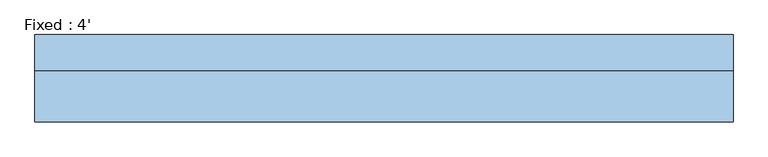
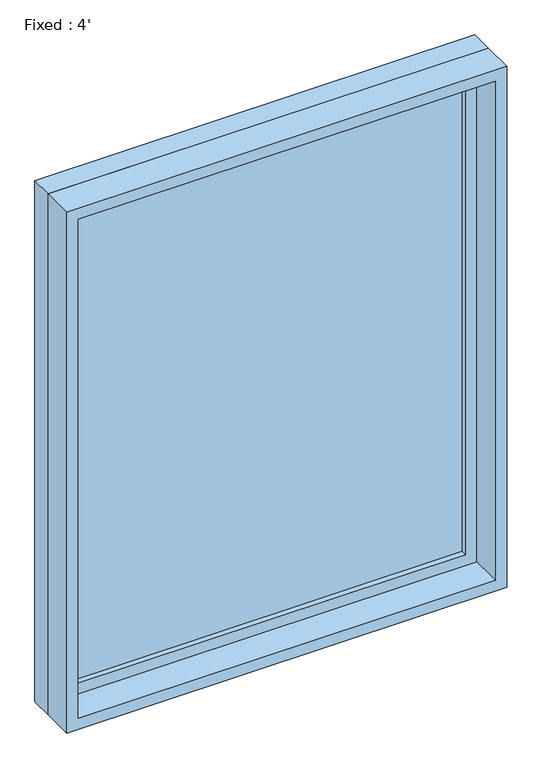
"""IFC4 building model written with IfcOpenShell, lengths in millimetres: window geometry, Fixed : 4'."""

from ifc_helpers import new_model, si_unit, frame, origin, place, context, project, spatial, polyline, outline, extrude, source, transform, mapped, element, save


def fixed_4_86eadd64(model_context):
    return source(origin(), model_context, "Body", "SweptSolid", [
        extrude(outline(polyline([(508.0, 28.575), (-584.2, 28.575), (-584.2, 41.275), (508.0, 41.275), (508.0, 28.575)])), frame((0.0, 0.0, 673.1), z_axis=(0.0, 0.0, 1.0), x_axis=(1.0, 0.0, 0.0)), (0.0, 0.0, 1.0), 1397.0),
        extrude(outline(polyline([(2114.55, -628.65), (628.65, -628.65), (628.65, 552.45), (2114.55, 552.45), (2114.55, -628.65)]), holes=[polyline([(2070.1, -584.2), (2070.1, 508.0), (673.1, 508.0), (673.1, -584.2), (2070.1, -584.2)])]), frame((0.0, 12.7, 0.0), z_axis=(0.0, 1.0, 0.0), x_axis=(0.0, 0.0, 1.0)), (0.0, 0.0, 1.0), 44.45),
        extrude(outline(polyline([(2133.6, -647.7), (609.6, -647.7), (609.6, 571.5), (2133.6, 571.5), (2133.6, -647.7)]), holes=[polyline([(2101.85, -615.95), (2101.85, 539.75), (641.35, 539.75), (641.35, -615.95), (2101.85, -615.95)])]), frame((0.0, -76.2, 0.0), z_axis=(0.0, 1.0, 0.0), x_axis=(0.0, 0.0, 1.0)), (0.0, 0.0, 1.0), 88.9),
        extrude(outline(polyline([(2133.6, 571.5), (2133.6, -647.7), (609.6, -647.7), (609.6, 571.5), (2133.6, 571.5)]), holes=[polyline([(2114.55, 552.45), (628.65, 552.45), (628.65, -628.65), (2114.55, -628.65), (2114.55, 552.45)])]), frame((0.0, 12.7, 0.0), z_axis=(0.0, 1.0, 0.0), x_axis=(0.0, 0.0, 1.0)), (0.0, 0.0, 1.0), 63.5),
    ])


if __name__ == "__main__":
    model = new_model("IFC4")
    model_context = context("Model", 3, world=origin())
    ifc_project = project(units=[si_unit("LENGTHUNIT", "METRE", prefix="MILLI")], contexts=[model_context])
    site = spatial("IfcSite", under=ifc_project)
    building = spatial("IfcBuilding", under=site)
    placement = place(None, origin())
    fixed_4_shape = fixed_4_86eadd64(model_context)
    element("IfcWindow", 1, ObjectType="Fixed : 4'", at=placement, inside=building, context=model_context, shape_type="MappedRepresentation", body=[
        mapped(fixed_4_shape, transform((0.0, 0.0, 0.0), x_axis=(1.0, 0.0, 0.0), y_axis=(0.0, 1.0, 0.0), z_axis=(0.0, 0.0, 1.0))),
    ])
    save(model, "model.ifc")

# Revit data of these elements
# Type "Fixed : 4'"
#   Type Mark = "13"
#   Construction Type Id = "GSP4R"
#   Assembly Code = "B2020100"
#   Analytic Construction = "1/8 in Pilkington single glazing"
#   Visual Light Transmittance = 0.9
#   Solar Heat Gain Coefficient = 0.78
#   Heat Transfer Coefficient (U) = 0.6496 BTU/(h·ft²·°F)
#   Height = 5' - 0"
#   Default Sill Height = 2' - 0"
#   Width = 4' - 0"
#   Window Inset = 0' - 0 3/4"
#   Define Thermal Properties by = 1
#   Glass Pane Material = Glass
#   Sash Material = Sash
#   Wall Closure = (empty or 0)
# Element 1 (IfcWindow, "Fixed : 4'")
#   Materials on its faces: "Sash", "Glass"
# Materials
#   "Glass": class "Glass", colour RGB 0 128 192, transparency 0.75, Description = "Soda Lime Glass", Cost = 0
#   "Sash": class "Wood", colour RGB 224 178 126, transparency 0
